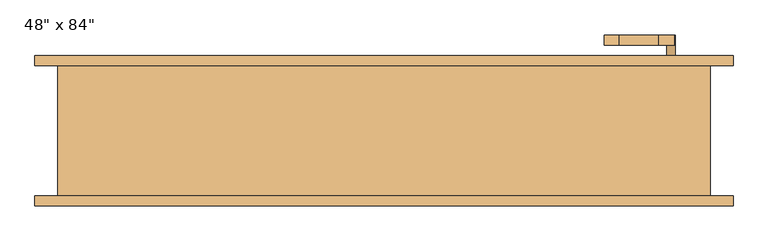
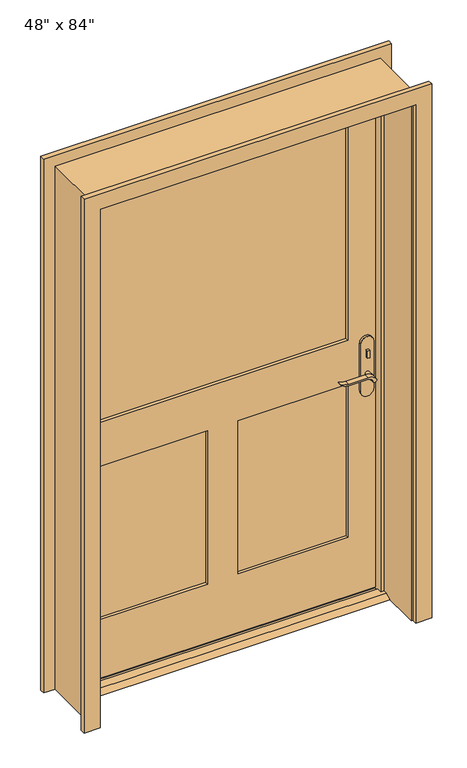
"""IFC4 building model written with IfcOpenShell, lengths in millimetres: door geometry."""

from ifc_helpers import new_model, si_unit, point, frame, frame_2d, origin, place, context, project, spatial, polyline, circle_curve, trimmed, segment, composite_curve, outline, extrude, faceted_brep, source, transform, mapped, element, save


def door_43baca08(model_context):
    return source(origin(), model_context, "Body", "SolidModel", [
        extrude(outline(polyline([(38.1, 12.7), (73.025, 12.7), (98.425, 0.0), (12.7, 0.0), (38.1, 12.7)])), frame((-609.6, 0.0, 0.0), z_axis=(1.0, 0.0, 0.0), x_axis=(0.0, 1.0, 0.0)), (0.0, 0.0, 1.0), 1219.2),
        extrude(outline(polyline([(563.8, 68.9), (553.8, 68.9), (553.8, 78.9), (563.8, 78.9), (563.8, 68.9)])), frame((0.0, 0.0, 981.9), z_axis=(0.0, 0.0, 1.0), x_axis=(1.0, 0.0, 0.0)), (0.0, 0.0, 1.0), 30.0),
        extrude(outline(composite_curve([segment(trimmed(circle_curve(frame_2d((996.9, 558.8)), 8.0), [point((996.9, 550.8))], [point((996.9, 566.8))], False, "CARTESIAN"), True, "CONTINUOUS"), segment(trimmed(circle_curve(frame_2d((996.9, 558.8)), 8.0), [point((996.9, 566.8))], [point((996.9, 550.8))], False, "CARTESIAN"), True, "CONTINUOUS")], self_intersect=False)), frame((0.0, 133.825, 0.0), z_axis=(0.0, 1.0, 0.0), x_axis=(0.0, 0.0, 1.0)), (0.0, 0.0, 1.0), 10.0),
        extrude(outline(composite_curve([segment(trimmed(circle_curve(frame_2d((897.1555521, 535.1324871)), 37.2832219), [point((919.0523287, 565.3081363))], [point((934.4, 533.4325667))], False, "CARTESIAN"), True, "CONTINUOUS"), segment(polyline([(934.4, 533.4325667), (934.4, 457.1564091)]), True, "CONTINUOUS"), segment(trimmed(circle_curve(frame_2d((1017.6850638, 457.2227909)), 83.2850902), [point((934.4, 457.1564091))], [point((939.4, 428.8))], True, "CARTESIAN"), True, "CONTINUOUS"), segment(polyline([(939.4, 428.8), (936.6135558, 428.8)]), True, "CONTINUOUS"), segment(trimmed(circle_curve(frame_2d((986.6709207, 460.7396612)), 59.3791355), [point((936.6135558, 428.8))], [point((927.4, 457.1564091))], False, "CARTESIAN"), True, "CONTINUOUS"), segment(polyline([(927.4, 457.1564091), (927.4, 533.4138099)]), True, "CONTINUOUS"), segment(trimmed(circle_curve(frame_2d((909.2738613, 533.4138099)), 18.1261387), [point((927.4, 533.4138099))], [point((914.4, 550.8))], True, "CARTESIAN"), True, "CONTINUOUS"), segment(trimmed(circle_curve(frame_2d((914.4, 558.8)), 8.0), [point((914.4, 550.8))], [point((919.0523287, 565.3081363))], False, "CARTESIAN"), True, "CONTINUOUS")], self_intersect=False)), frame((0.0, 28.9, 0.0), z_axis=(0.0, 1.0, 0.0), x_axis=(0.0, 0.0, 1.0)), (0.0, 0.0, 1.0), 20.0),
        extrude(outline(composite_curve([segment(trimmed(circle_curve(frame_2d((914.4, 558.8)), 8.0), [point((914.3999903, 550.8))], [point((919.0523287, 565.3081363))], False, "CARTESIAN"), True, "CONTINUOUS"), segment(trimmed(circle_curve(frame_2d((897.1555521, 535.1324871)), 37.2832219), [point((919.0523287, 565.3081363))], [point((934.4, 533.4325667))], False, "CARTESIAN"), True, "CONTINUOUS"), segment(polyline([(934.4, 533.4325667), (934.4, 457.1564091)]), True, "CONTINUOUS"), segment(trimmed(circle_curve(frame_2d((1017.6850638, 457.2227909)), 83.2850902), [point((934.4, 457.1564091))], [point((939.4, 428.8))], True, "CARTESIAN"), True, "CONTINUOUS"), segment(polyline([(939.4, 428.8), (936.6135558, 428.8)]), True, "CONTINUOUS"), segment(trimmed(circle_curve(frame_2d((986.6709207, 460.7396612)), 59.3791355), [point((936.6135558, 428.8))], [point((927.4, 457.1564091))], False, "CARTESIAN"), True, "CONTINUOUS"), segment(polyline([(927.4, 457.1564091), (927.4, 533.4138122)]), True, "CONTINUOUS"), segment(trimmed(circle_curve(frame_2d((909.2738682, 533.4138122)), 18.1261318), [point((927.4, 533.4138122))], [point((914.3999903, 550.8))], True, "CARTESIAN"), True, "CONTINUOUS")], self_intersect=False)), frame((0.0, 163.825, 0.0), z_axis=(0.0, 1.0, 0.0), x_axis=(0.0, 0.0, 1.0)), (0.0, 0.0, 1.0), 20.0),
        extrude(outline(composite_curve([segment(trimmed(circle_curve(frame_2d((914.4, 558.8)), 8.0), [point((914.4, 550.8))], [point((914.4, 566.8))], False, "CARTESIAN"), True, "CONTINUOUS"), segment(trimmed(circle_curve(frame_2d((914.4, 558.8)), 8.0), [point((914.4, 566.8))], [point((914.4, 550.8))], False, "CARTESIAN"), True, "CONTINUOUS")], self_intersect=False)), frame((0.0, 48.9, 0.0), z_axis=(0.0, 1.0, 0.0), x_axis=(0.0, 0.0, 1.0)), (0.0, 0.0, 1.0), 30.0),
        extrude(outline(composite_curve([segment(trimmed(circle_curve(frame_2d((914.4, 558.8)), 8.0), [point((914.4, 550.8))], [point((914.4, 566.8))], False, "CARTESIAN"), True, "CONTINUOUS"), segment(trimmed(circle_curve(frame_2d((914.4, 558.8)), 8.0), [point((914.4, 566.8))], [point((914.4, 550.8))], False, "CARTESIAN"), True, "CONTINUOUS")], self_intersect=False)), frame((0.0, 133.825, 0.0), z_axis=(0.0, 1.0, 0.0), x_axis=(0.0, 0.0, 1.0)), (0.0, 0.0, 1.0), 30.0),
        extrude(outline(composite_curve([segment(polyline([(844.4, 583.8), (1039.4, 583.8)]), True, "CONTINUOUS"), segment(trimmed(circle_curve(frame_2d((1039.4, 558.8)), 25.0), [point((1039.4, 583.8))], [point((1039.4, 533.8))], False, "CARTESIAN"), True, "CONTINUOUS"), segment(polyline([(1039.4, 533.8), (844.4, 533.8)]), True, "CONTINUOUS"), segment(trimmed(circle_curve(frame_2d((844.4, 558.8)), 25.0), [point((844.4, 533.8))], [point((844.4, 583.8))], False, "CARTESIAN"), True, "CONTINUOUS")], self_intersect=False)), frame((0.0, 78.9, 0.0), z_axis=(0.0, 1.0, 0.0), x_axis=(0.0, 0.0, 1.0)), (0.0, 0.0, 1.0), 10.0),
        extrude(outline(composite_curve([segment(polyline([(844.4, 583.8), (1039.4, 583.8)]), True, "CONTINUOUS"), segment(trimmed(circle_curve(frame_2d((1039.4, 558.8)), 25.0), [point((1039.4, 583.8))], [point((1039.4, 533.8))], False, "CARTESIAN"), True, "CONTINUOUS"), segment(polyline([(1039.4, 533.8), (844.4, 533.8)]), True, "CONTINUOUS"), segment(trimmed(circle_curve(frame_2d((844.4, 558.8)), 25.0), [point((844.4, 533.8))], [point((844.4, 583.8))], False, "CARTESIAN"), True, "CONTINUOUS")], self_intersect=False)), frame((0.0, 123.825, 0.0), z_axis=(0.0, 1.0, 0.0), x_axis=(0.0, 0.0, 1.0)), (0.0, 0.0, 1.0), 10.0),
        faceted_brep([(635.0, 123.825, 0.0), (635.0, -130.175, 0.0), (609.6, -130.175, 0.0), (609.6, 53.975, 0.0), (596.9, 53.975, 0.0), (596.9, 88.9, 0.0), (609.6, 88.9, 0.0), (609.6, 123.825, 0.0), (635.0, 123.825, 2159.0), (635.0, -130.175, 2159.0), (-635.0, -130.175, 2159.0), (-635.0, -130.175, 0.0), (-609.6, -130.175, 0.0), (-609.6, -130.175, 2133.6), (609.6, -130.175, 2133.6), (609.6, 53.975, 2133.6), (-609.6, 53.975, 2133.6), (-609.6, 53.975, 0.0), (-596.9, 53.975, 0.0), (-596.9, 53.975, 2120.9), (596.9, 53.975, 2120.9), (596.9, 88.9, 2120.9), (-596.9, 88.9, 2120.9), (-596.9, 88.9, 0.0), (-609.6, 88.9, 0.0), (-609.6, 88.9, 2133.6), (609.6, 88.9, 2133.6), (609.6, 123.825, 2133.6), (-609.6, 123.825, 2133.6), (-609.6, 123.825, 0.0), (-635.0, 123.825, 0.0), (-635.0, 123.825, 2159.0)], [[[0, 1, 2, 3, 4, 5, 6, 7]], [[1, 0, 8, 9]], [[2, 1, 9, 10, 11, 12, 13, 14]], [[3, 2, 14, 15]], [[4, 3, 15, 16, 17, 18, 19, 20]], [[5, 4, 20, 21]], [[6, 5, 21, 22, 23, 24, 25, 26]], [[7, 6, 26, 27]], [[0, 7, 27, 28, 29, 30, 31, 8]], [[9, 8, 31, 10]], [[15, 14, 13, 16]], [[21, 20, 19, 22]], [[27, 26, 25, 28]], [[30, 29, 24, 23, 18, 17, 12, 11]], [[10, 31, 30, 11]], [[16, 13, 12, 17]], [[22, 19, 18, 23]], [[28, 25, 24, 29]]]),
        extrude(outline(polyline([(2133.6, -609.6), (12.7, -609.6), (12.7, 609.6), (2133.6, 609.6), (2133.6, -609.6)]), holes=[polyline([(1066.8, -488.95), (2012.95, -488.95), (2012.95, 488.95), (1066.8, 488.95), (1066.8, -488.95)]), polyline([(885.825, -60.325), (254.0, -60.325), (254.0, -488.95), (885.825, -488.95), (885.825, -60.325)]), polyline([(885.825, 488.95), (254.0, 488.95), (254.0, 60.325), (885.825, 60.325), (885.825, 488.95)])]), frame((0.0, 88.9, 0.0), z_axis=(0.0, 1.0, 0.0), x_axis=(0.0, 0.0, 1.0)), (0.0, 0.0, 1.0), 34.925),
        extrude(outline(polyline([(488.95, 102.87), (-488.95, 102.87), (-488.95, 109.855), (488.95, 109.855), (488.95, 102.87)])), frame((0.0, 0.0, 1066.8), z_axis=(0.0, 0.0, 1.0), x_axis=(1.0, 0.0, 0.0)), (0.0, 0.0, 1.0), 946.15),
        extrude(outline(polyline([(-60.325, 100.5416667), (-488.95, 100.5416667), (-488.95, 112.1833333), (-60.325, 112.1833333), (-60.325, 100.5416667)])), frame((0.0, 0.0, 254.0), z_axis=(0.0, 0.0, 1.0), x_axis=(1.0, 0.0, 0.0)), (0.0, 0.0, 1.0), 631.825),
        extrude(outline(polyline([(488.95, 100.5416667), (60.325, 100.5416667), (60.325, 112.1833333), (488.95, 112.1833333), (488.95, 100.5416667)])), frame((0.0, 0.0, 254.0), z_axis=(0.0, 0.0, 1.0), x_axis=(1.0, 0.0, 0.0)), (0.0, 0.0, 1.0), 631.825),
        extrude(outline(polyline([(0.0, -679.45), (0.0, -615.95), (2139.95, -615.95), (2139.95, 615.95), (0.0, 615.95), (0.0, 679.45), (2203.45, 679.45), (2203.45, -679.45), (0.0, -679.45)])), frame((0.0, 123.825, 0.0), z_axis=(0.0, 1.0, 0.0), x_axis=(0.0, 0.0, 1.0)), (0.0, 0.0, 1.0), 19.05),
        extrude(outline(polyline([(0.0, -679.45), (0.0, -615.95), (2139.95, -615.95), (2139.95, 615.95), (0.0, 615.95), (0.0, 679.45), (2203.45, 679.45), (2203.45, -679.45), (0.0, -679.45)])), frame((0.0, -149.225, 0.0), z_axis=(0.0, 1.0, 0.0), x_axis=(0.0, 0.0, 1.0)), (0.0, 0.0, 1.0), 19.05),
    ])


if __name__ == "__main__":
    model = new_model("IFC4")
    model_context = context("Model", 3, world=origin())
    ifc_project = project(units=[si_unit("LENGTHUNIT", "METRE", prefix="MILLI")], contexts=[model_context])
    site = spatial("IfcSite", under=ifc_project)
    building = spatial("IfcBuilding", under=site)
    placement = place(None, origin())
    door_shape = door_43baca08(model_context)
    element("IfcDoor", 1, ObjectType="48\" x 84\"", at=placement, inside=building, context=model_context, shape_type="MappedRepresentation", body=[
        mapped(door_shape, transform((0.0, 0.0, 0.0), x_axis=(1.0, 0.0, 0.0), y_axis=(0.0, 1.0, 0.0), z_axis=(0.0, 0.0, 1.0))),
    ])
    save(model, "model.ifc")

# Revit data of these elements
# Type "48\" x 84\""
#   Type Mark = "14"
#   Assembly Code = "B2030100"
#   Analytic Construction = "French door, wood frame with single glass"
#   Top Rail = 0' - 4 3/4"
#   Threshold Offset [instance default] = 0' - 0 1/2"
#   Thickness = 0' - 1 3/8"
#   Thermal Resistance (R) = 1.0696 (h·ft²·°F)/BTU
#   Swing Angle [instance default] = 90.00°
#   Stiles = 0' - 4 3/4"
#   Rough Width = 4' - 2"
#   Rough Height = 7' - 1"
#   Lock Rail = 0' - 7 1/8"
#   Height = 7' - 0"
#   Width = 4' - 0"
#   Heat Transfer Coefficient (U) = 0.9350 BTU/(h·ft²·°F)
#   Door Offset [instance default] = 0' - 0"
#   Bottom Rail = 0' - 9 1/2"
#   Threshold [instance default] = yes
#   Function = 1
#   Exterior Trim [instance default] = yes
#   Trim Material = Cherry
#   Threshold Material = Cherry
#   Panel Material = Cherry
#   Glazing = Glass
#   Frame Material = Cherry
#   Door Handle Material = Aluminum
#   Visual Light Transmittance = 0
#   Solar Heat Gain Coefficient = 0
#   Wall Closure = (empty or 0)
#   Construction Type = (empty or 0)
# Element 1 (IfcDoor, "48\" x 84\"")
#   Materials on its faces: "Cherry", "Aluminum", "Glass"
# Materials
#   "Cherry": class "Wood", colour RGB 226 177 128, transparency 0, Description = "Prunus Serotina", Cost = 0
#   "Glass": class "Glass", colour RGB 0 128 192, transparency 0.75, Description = "Soda Lime Glass", Cost = 0
#   "Aluminum": class "Metal", colour RGB 247 247 247, transparency 0, Description = "Aluminum 6061", Cost = 0
